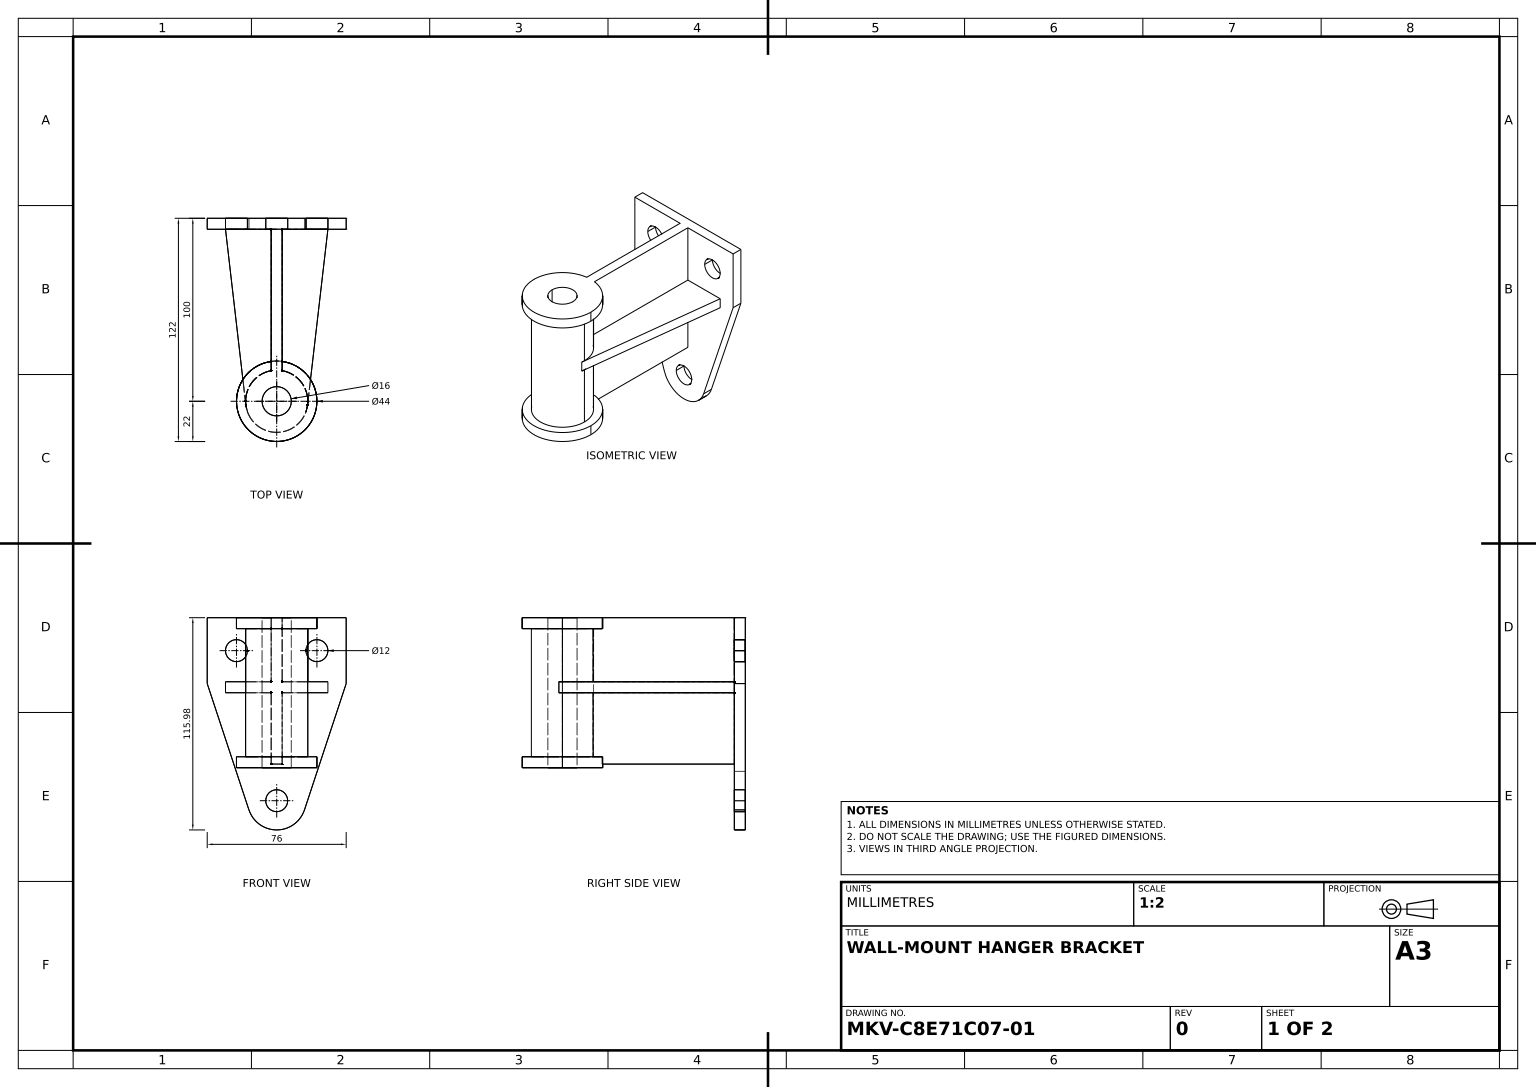
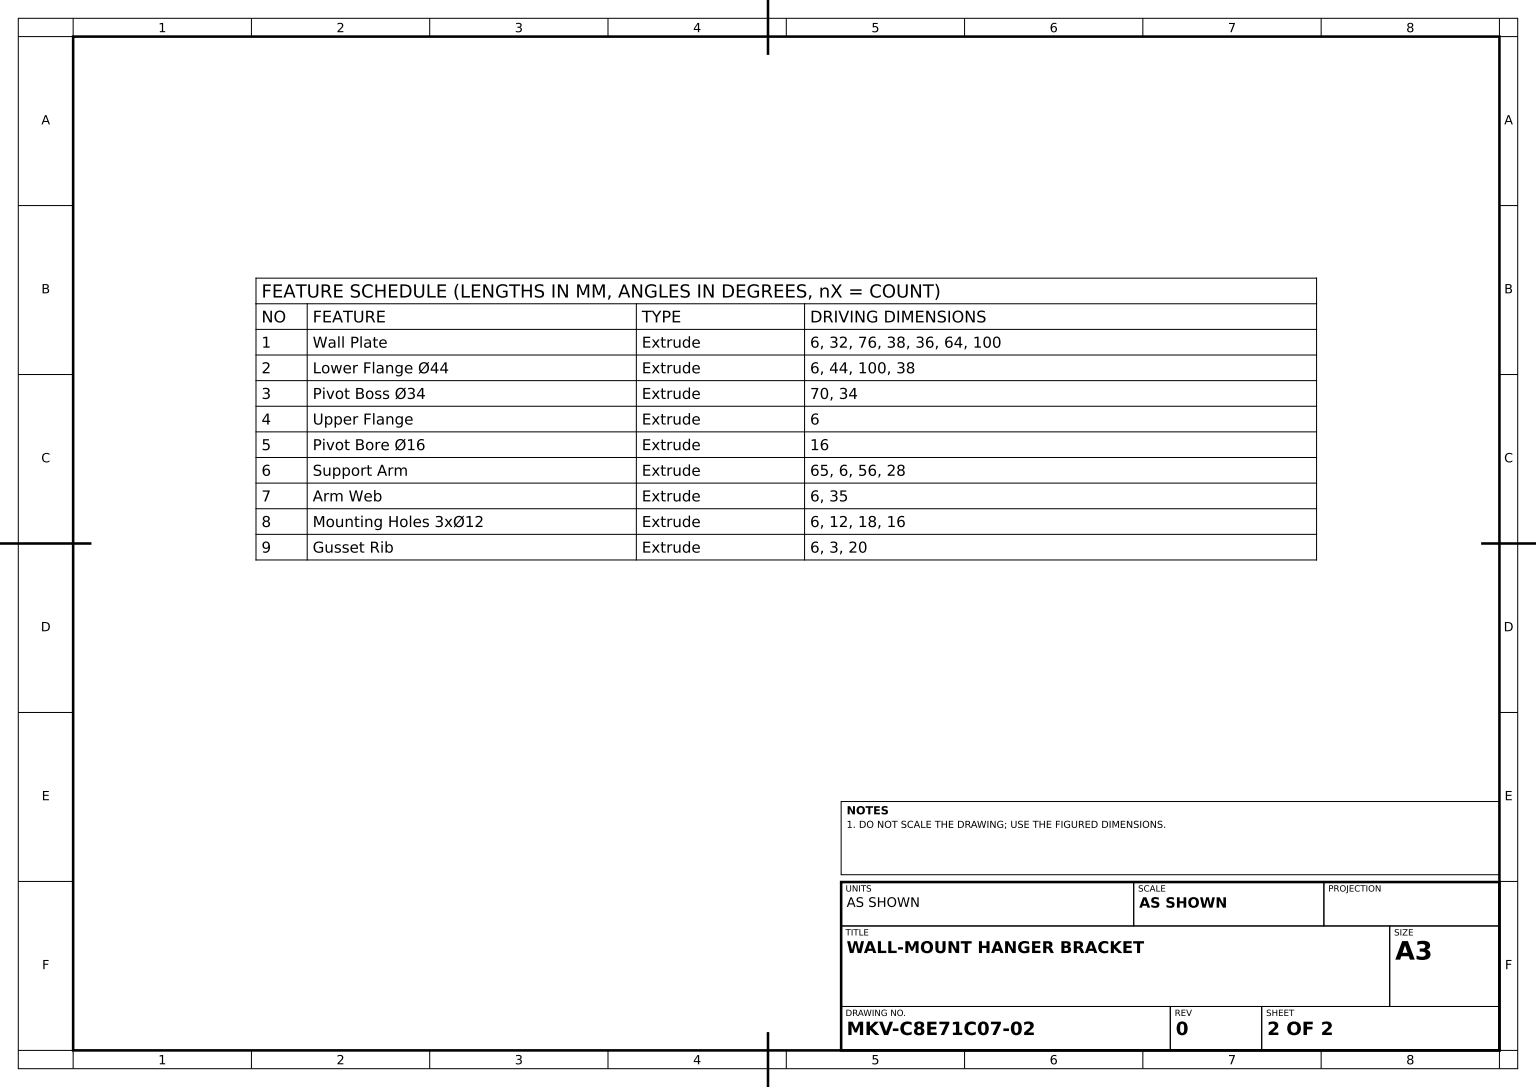
from build123d import *

# Parameters (mm, degrees)
WALL_PLATE_DEPTH           = 6
LOWER_FLANGE_SKETCH_R      = 22
LOWER_FLANGE_44_DEPTH      = 6
PIVOT_BOSS_SKETCH_R        = 17
PIVOT_BOSS_34_DEPTH        = 70
UPPER_FLANGE_SKETCH_R      = 22
UPPER_FLANGE_DEPTH         = 6
PIVOT_BORE_SKETCH_R        = 8
PIVOT_BORE_16_DEPTH        = 173.580416038
SUPPORT_ARM_DEPTH          = 6
ARM_WEB_REACH              = 159.797
ARM_WEB_SKETCH_W           = 6
ARM_WEB_SKETCH_H           = 35
MOUNTING_HOLES_SKETCH_R    = 6
MOUNTING_HOLES_3X_12_DEPTH = 6
GUSSET_RIB_REACH           = 159.797
GUSSET_RIB_SKETCH_W        = 6
GUSSET_RIB_SKETCH_H        = 39


with BuildPart() as part:
    # Wall Plate Sketch → Wall Plate (new body)
    with BuildSketch(Plane.XY):
        with BuildLine():
            Line((-38, 64), (-15.192006216, -5.020253691))
            ThreePointArc((-15.192006216, -5.020253691), (0, -16), (15.192006216, -5.020253691))
            Line((15.192006216, -5.020253691), (38, 64))
            Line((38, 64), (38, 100))
            Line((38, 100), (-38, 100))
            Line((-38, 100), (-38, 64))
        make_face()
    extrude(amount=WALL_PLATE_DEPTH)



with BuildPart() as body_2:
    # Lower Flange Sketch → Lower Flange Ø44 (new body)
    with BuildSketch(Plane(origin=(0, 100, 0), x_dir=(1, 0, 0), z_dir=(0, 1, 0))):
        with Locations(Location((0, -100, 0), (0, 0, 180))):
            Circle(LOWER_FLANGE_SKETCH_R)
    extrude(amount=-LOWER_FLANGE_44_DEPTH)

    # Pivot Boss Sketch → Pivot Boss Ø34 (add)
    with BuildSketch(Plane.XZ.offset(-94)):
        with Locations((0, 100)):
            Circle(PIVOT_BOSS_SKETCH_R)
    extrude(amount=PIVOT_BOSS_34_DEPTH)

    # Upper Flange Sketch → Upper Flange (add)
    with BuildSketch(Plane.XZ.offset(-24)):
        with Locations(Location((0, 100, 0), (0, 0, 180))):
            Circle(UPPER_FLANGE_SKETCH_R)
    extrude(amount=UPPER_FLANGE_DEPTH)

    # Pivot Bore Sketch → Pivot Bore Ø16 (cut, through all)
    with BuildSketch(Plane(origin=(0, 100, 0), x_dir=(1, 0, 0), z_dir=(0, 1, 0))):
        with Locations(Location((0, -100, 0), (0, 0, 180))):
            Circle(PIVOT_BORE_SKETCH_R)
    extrude(amount=-PIVOT_BORE_16_DEPTH, mode=Mode.SUBTRACT)


with BuildPart() as part_1:
    add(part.part)

    add(body_2.part)  # Support Arm merges body 2
    # Support Arm Sketch → Support Arm (add)
    with BuildSketch(Plane(origin=(0, 65, 0), x_dir=(1, 0, 0), z_dir=(0, 1, 0))):
        with BuildLine():
            Line((-28, -6), (28, -6))
            Line((28, -6), (16.887127656, -101.955740153))
            ThreePointArc((16.887127656, -101.955740153), (0, -83), (-16.887127656, -101.955740153))
            Line((-16.887127656, -101.955740153), (-28, -6))
        make_face()
    extrude(amount=-SUPPORT_ARM_DEPTH)

    # Arm Web Sketch → Arm Web (add, up to next)
    with BuildSketch(Plane.XY.offset(6), mode=Mode.PRIVATE) as arm_web_sk1:
        with Locations((0, 82.5)):
            Rectangle(ARM_WEB_SKETCH_W, ARM_WEB_SKETCH_H)
    arm_web_tool1 = extrude(arm_web_sk1.sketch, amount=ARM_WEB_REACH, mode=Mode.PRIVATE) - part_1.part
    add(arm_web_tool1.solids().sort_by_distance((0, 82.5, 6))[0])

    # Mounting Holes Sketch → Mounting Holes 3xØ12 (cut)
    with BuildSketch(Plane.XY.offset(6)):
        Circle(MOUNTING_HOLES_SKETCH_R)
        with Locations((-22, 82)):
            Circle(MOUNTING_HOLES_SKETCH_R)
        with Locations((22, 82)):
            Circle(MOUNTING_HOLES_SKETCH_R)
    extrude(amount=-MOUNTING_HOLES_3X_12_DEPTH, mode=Mode.SUBTRACT)

    # Gusset Rib Sketch → Gusset Rib (add, up to next)
    with BuildSketch(Plane.XY.offset(6), mode=Mode.PRIVATE) as gusset_rib_sk1:
        with Locations((0, 39.5)):
            Rectangle(GUSSET_RIB_SKETCH_W, GUSSET_RIB_SKETCH_H)
    gusset_rib_tool1 = extrude(gusset_rib_sk1.sketch, amount=GUSSET_RIB_REACH, mode=Mode.PRIVATE) - part_1.part
    add(gusset_rib_tool1.solids().sort_by_distance((0, 39.5, 6))[0])


solid = part_1.part
